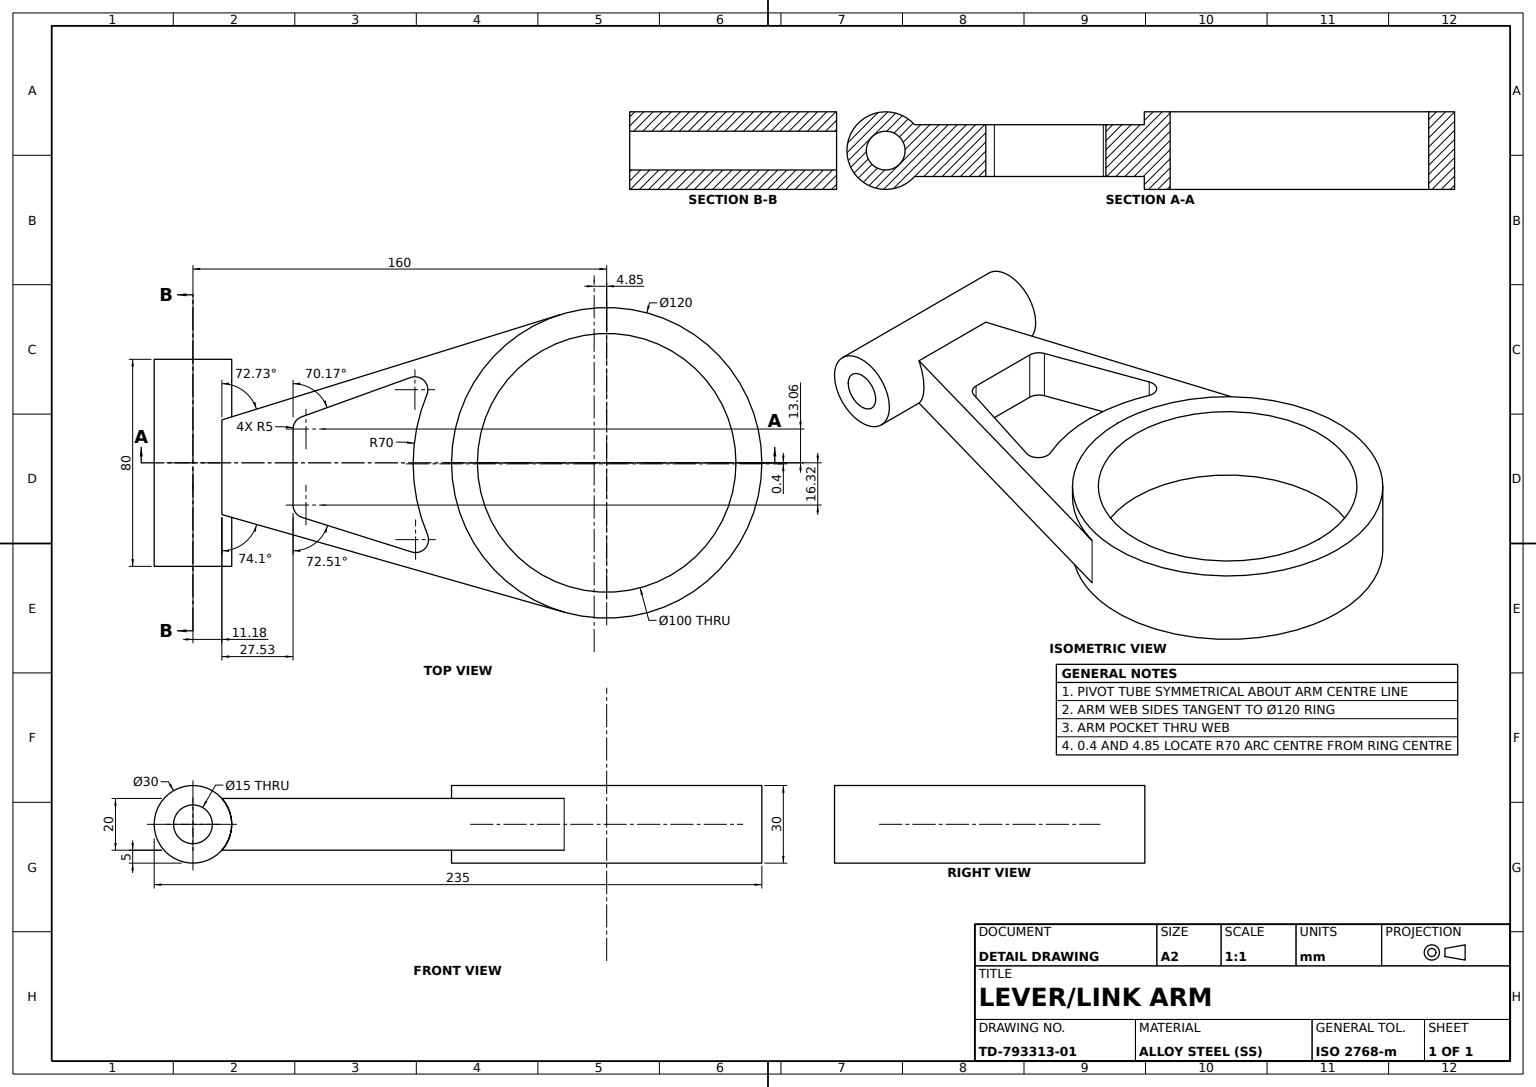
from build123d import *

# Parameters (mm, degrees)
PIVOT_TUBE_SKETCH_R         = 15
PIVOT_TUBE_SKETCH_R_2       = 7.5
PIVOT_TUBE_30X_15_DEPTH     = 40
ARM_WEB_20MM_DEPTH          = 10
RING_HUB_SKETCH_R           = 60
RING_HUB_SKETCH_R_2         = 50
RING_HUB_120X_100_DEPTH     = 15
ARM_LIGHTENING_POCKET_DEPTH = 230.401394939


with BuildPart() as part:
    # Pivot Tube Sketch → Pivot Tube Ø30xØ15 (new, symmetric)
    with BuildSketch(Plane(origin=(0, 0, 0), x_dir=(0, 0, -1), z_dir=(1, 0, 0))):
        Circle(PIVOT_TUBE_SKETCH_R)
        Circle(PIVOT_TUBE_SKETCH_R_2, mode=Mode.SUBTRACT)
    extrude(amount=PIVOT_TUBE_30X_15_DEPTH, both=True)

    # Arm Web Sketch → Arm Web 20mm (add, symmetric)
    with BuildSketch(Plane(origin=(0, 0, 0), x_dir=(1, 0, 0), z_dir=(0, 1, 0))):
        with BuildLine():
            Line((-57.295515099, 142.189218166), (-16.443257741, 10.771566203))
            Line((-16.443257741, 10.771566203), (19.870461321, 10.771566203))
            Line((19.870461321, 10.771566203), (57.703615224, 143.559416372))
            ThreePointArc((57.703615224, 143.559416372), (0.714840688, 100.004258461), (-57.295515099, 142.189218166))
        make_face()
    extrude(amount=ARM_WEB_20MM_DEPTH, both=True)

    # Ring Hub Sketch → Ring Hub Ø120xØ100 (add, symmetric)
    with BuildSketch(Plane(origin=(0, 0, 0), x_dir=(1, 0, 0), z_dir=(0, 1, 0))):
        with Locations(Location((0, 160, 0), (0, 0, 270))):
            Circle(RING_HUB_SKETCH_R)
        with Locations(Location((0, 160, 0), (0, 0, 270))):
            Circle(RING_HUB_SKETCH_R_2, mode=Mode.SUBTRACT)
    extrude(amount=RING_HUB_120X_100_DEPTH, both=True)

    # Arm Pocket Sketch → Arm Lightening Pocket (cut, through all)
    with BuildSketch(Plane(origin=(0, 10, 0), x_dir=(1, 0, 0), z_dir=(0, 1, 0))):
        with BuildLine():
            Line((-13.0584069, 38.71360492), (16.320169694, 38.71360492))
            ThreePointArc((16.320169694, 38.71360492), (19.277035427, 39.681614712), (21.088991166, 42.210826904))
            Line((21.088991166, 42.210826904), (34.445867452, 84.596700091))
            ThreePointArc((34.445867452, 84.596700091), (33.039335954, 89.800154549), (27.725249342, 90.702791032))
            ThreePointArc((27.725249342, 90.702791032), (0.71662682, 85.149887641), (-26.34110962, 90.458307872))
            ThreePointArc((-26.34110962, 90.458307872), (-31.704790858, 89.453148124), (-32.954629394, 84.141149802))
            Line((-32.954629394, 84.141149802), (-17.761840528, 42.017222858))
            ThreePointArc((-17.761840528, 42.017222858), (-15.932262297, 39.622033687), (-13.0584069, 38.71360492))
        make_face()
    extrude(amount=-ARM_LIGHTENING_POCKET_DEPTH, mode=Mode.SUBTRACT)


solid = part.part
